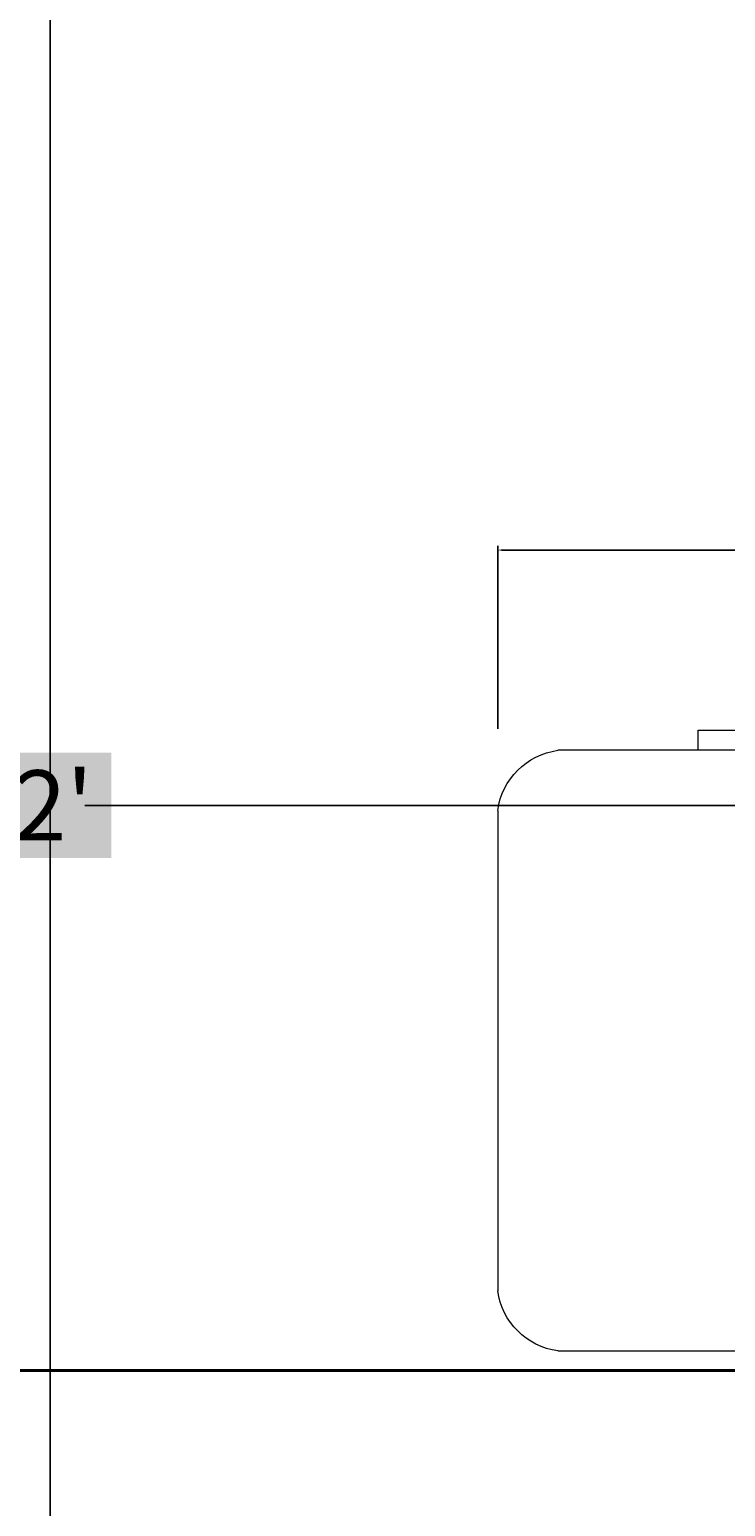
# Model space of a CAD drawing. Units: inches. Extents: x -301 to 715, y -607 to 364.
# Tile 77 of 141: x -123 to -94, y -73 to -10. Entities that reach past the tile are written whole.
import ezdxf

# ---------------------------------------------------------------- set-up
doc = ezdxf.new("R2010")
doc.units = ezdxf.units.IN
doc.header["$MEASUREMENT"] = 0
for name, color, linetype, lineweight in [('A-ANNO-DIMS', 2, 'Continuous', 18), ('A-FURN', 8, 'Continuous', 18), ('A-WALL', 3, 'Continuous', 40)]:
    doc.layers.add(name, color=color, linetype=linetype, lineweight=lineweight)
doc.styles.get("Standard").update_dxf_attribs({"font": 'arial.ttf'})
doc.dimstyles.get("Standard").update_dxf_attribs({"dimtxt": 0.18, "dimasz": 0.18, "dimexe": 0.18, "dimexo": 0.0625, "dimgap": 0.09, "dimtad": 0, "dimtih": 1, "dimtoh": 1, "dimdec": 1, "dimzin": 0, "dimdsep": 46, "dimlunit": 4, "dimtxsty": 'Standard', "dimcen": 0.09, "dimclrd": 3, "dimclre": 4, "dimclrt": 6, "dimadec": 0, "dimazin": 0, "dimtfac": 1, "dimtdec": 1, "dimtofl": 0, "dimtmove": 0, "dimatfit": 3, "dimfxl": 1, "dimtfill": 2, "dimtfillclr": 51, "dimtolj": 1, "dimtzin": 0, "dimarcsym": 0})

# ---------------------------------------------------------------- blocks, each defined once
blk = doc.blocks.new('Desk - 30 x 60 in.')
for p, q in [((-26.999995, 0), (26.999995, 0)), ((-29.999995, -27), (-29.999995, -3)), ((29.999995, -3), (29.999995, -27)), ((26.999995, -30), (-26.999995, -30)), ((-20.000005, -30), (-20.000005, -31)), ((-16.000005, -31), (-16.000005, -30)), ((15.999995, -31), (15.999995, -30)), ((19.999995, -30), (19.999995, -31)), ((-20.000005, -31), (-16.000005, -31)), ((19.999995, -31), (15.999995, -31))]:
    blk.add_line(p, q)
for centre, start, end in [((-26.499995, -3.5), 98.1301, 171.8699), ((26.499995, -3.5), 8.130102, 81.8699), ((-26.499995, -26.5), 188.1301, 261.8699), ((26.499995, -26.5), 278.1301, 351.8699)]:
    blk.add_arc(centre, 3.535534, start, end)
blk = doc.blocks.new('*D57')
at = {"layer": 'A-ANNO-DIMS', "color": 0, "lineweight": -2, "transparency": 16777216}
for p, q in [((-195.603, -67.255), (-195.603, -42.99)), ((-190.603, -43.17), (-126.098, -43.17)), ((-56.603, -43.17), (-121.109, -43.17)), ((-51.603, -67.255), (-51.603, -42.99))]:
    blk.add_line(p, q, dxfattribs=at)
at = {"layer": 'A-ANNO-DIMS', "color": 0, "transparency": 16777216}
for points in [[(-190.603, -42.336), (-190.603, -44.003), (-195.603, -43.17)], [(-56.603, -42.336), (-56.603, -44.003), (-51.603, -43.17)]]:
    blk.add_solid(points, dxfattribs=at)
at = {"layer": 'Defpoints', "color": 0, "transparency": 16777216}
for p in [(-51.603, -43.17), (-195.603, -67.318), (-51.603, -67.318)]:
    blk.add_point(p, dxfattribs=at)
at = {"layer": 'A-ANNO-DIMS', "color": 0, "transparency": 16777216, "insert": (-123.603, -43.17), "char_height": 3, "attachment_point": 5, "bg_fill": 1, "box_fill_scale": 1.25, "bg_fill_color": 51, "bg_fill_transparency": 0}
blk.add_mtext("\\A1;12'", dxfattribs=at)
blk = doc.blocks.new('*D114')
at = {"layer": 'A-ANNO-DIMS', "color": 4, "lineweight": -2, "transparency": 16777216}
for p, q in [((-103.477, -39.895), (-103.477, -32.076)), ((-52.128, -39.895), (-52.128, -32.076))]:
    blk.add_line(p, q, dxfattribs=at)
at = {"layer": 'A-ANNO-DIMS', "color": 3, "lineweight": -2, "transparency": 16777216}
for p, q in [((-103.297, -32.256), (-79.024, -32.256)), ((-52.308, -32.256), (-76.581, -32.256))]:
    blk.add_line(p, q, dxfattribs=at)
at = {"layer": 'A-ANNO-DIMS', "color": 3, "transparency": 16777216}
for points in [[(-103.297, -32.226), (-103.297, -32.286), (-103.477, -32.256)], [(-52.308, -32.226), (-52.308, -32.286), (-52.128, -32.256)]]:
    blk.add_solid(points, dxfattribs=at)
at = {"layer": 'Defpoints', "color": 0, "transparency": 16777216}
for p in [(-52.128, -32.256), (-103.477, -39.958), (-52.128, -39.958)]:
    blk.add_point(p, dxfattribs=at)
at = {"layer": 'A-ANNO-DIMS', "color": 6, "transparency": 16777216, "insert": (-77.803, -32.256), "char_height": 0.18, "attachment_point": 5, "bg_fill": 1, "box_fill_scale": 1.25, "bg_fill_color": 51, "bg_fill_transparency": 0}
blk.add_mtext('\\A1;DESK 4\'-3 1/2" TYP.', dxfattribs=at)
blk = doc.blocks.new('*D151')
at = {"layer": 'A-ANNO-DIMS', "color": 4, "lineweight": -2, "transparency": 16777216}
for p, q in [((-204.603, -223.755), (-204.603, 359.612)), ((-45.603, -214.755), (-45.603, 359.612))]:
    blk.add_line(p, q, dxfattribs=at)
at = {"layer": 'A-ANNO-DIMS', "color": 3, "lineweight": -2, "transparency": 16777216}
for p, q in [((-204.423, 359.432), (-125.494, 359.432)), ((-45.783, 359.432), (-124.713, 359.432))]:
    blk.add_line(p, q, dxfattribs=at)
at = {"layer": 'A-ANNO-DIMS', "color": 3, "transparency": 16777216}
for points in [[(-204.423, 359.462), (-204.423, 359.402), (-204.603, 359.432)], [(-45.783, 359.462), (-45.783, 359.402), (-45.603, 359.432)]]:
    blk.add_solid(points, dxfattribs=at)
at = {"layer": 'Defpoints', "color": 0, "transparency": 16777216}
for p in [(-45.603, 359.432), (-45.603, -214.818), (-204.603, -223.818)]:
    blk.add_point(p, dxfattribs=at)
at = {"layer": 'A-ANNO-DIMS', "color": 6, "transparency": 16777216, "insert": (-125.103, 359.432), "char_height": 0.18, "attachment_point": 5, "bg_fill": 1, "box_fill_scale": 1.25, "bg_fill_color": 51, "bg_fill_transparency": 0}
blk.add_mtext('\\A1;13\'-3"', dxfattribs=at)
blk = doc.blocks.new('*D158')
at = {"layer": 'A-ANNO-DIMS', "color": 4, "lineweight": -2, "transparency": 16777216}
for p, q in [((-122.603, 221.62), (-122.603, -296.865)), ((-50.603, 221.62), (-50.603, -296.865))]:
    blk.add_line(p, q, dxfattribs=at)
at = {"layer": 'A-ANNO-DIMS', "color": 3, "lineweight": -2, "transparency": 16777216}
for p, q in [((-122.423, -296.685), (-86.933, -296.685)), ((-50.783, -296.685), (-86.274, -296.685))]:
    blk.add_line(p, q, dxfattribs=at)
at = {"layer": 'A-ANNO-DIMS', "color": 3, "transparency": 16777216}
for points in [[(-122.423, -296.655), (-122.423, -296.715), (-122.603, -296.685)], [(-50.783, -296.655), (-50.783, -296.715), (-50.603, -296.685)]]:
    blk.add_solid(points, dxfattribs=at)
at = {"layer": 'Defpoints', "color": 0, "transparency": 16777216}
for p in [(-122.603, 221.682), (-50.603, 221.682), (-50.603, -296.685)]:
    blk.add_point(p, dxfattribs=at)
at = {"layer": 'A-ANNO-DIMS', "color": 6, "transparency": 16777216, "insert": (-86.603, -296.685), "char_height": 0.18, "attachment_point": 5, "bg_fill": 1, "box_fill_scale": 1.25, "bg_fill_color": 51, "bg_fill_transparency": 0}
blk.add_mtext('\\A1;6\'-0"', dxfattribs=at)

msp = doc.modelspace()

# ---------------------------------------------------------------- linework, layer by layer
at = {"layer": 'A-WALL'}
msp.add_line((-195.603, -67.318), (-51.603, -67.318), dxfattribs=at)

# ---------------------------------------------------------------- block references
at = {"layer": 'A-FURN', "xscale": -0.8558048107780498, "yscale": 0.8558048107780498, "zscale": 0.8558048107780498, "rotation": 180}
msp.add_blockref('Desk - 30 x 60 in.', (-77.803, -66.488), dxfattribs=at)

# ---------------------------------------------------------------- dimensions: what is measured, and where the dimension line sits
at = {"layer": 'A-ANNO-DIMS'}
for base, p1, p2, override, picture, middle in [((-45.603, 359.432), (-204.603, -223.818), (-45.603, -214.818), {"dimdec": 1, "dimlfac": 1, "dimrnd": 0, "dimzin": 1, "dimdsep": 46, "dimlunit": 4, "dimfrac": 2}, '*D151', (-125.103, 359.432)), ((-50.603, -296.685), (-122.603, 221.682), (-50.603, 221.682), {"dimdec": 1, "dimlfac": 1, "dimrnd": 0, "dimzin": 1, "dimdsep": 46, "dimlunit": 4, "dimfrac": 2}, '*D158', (-86.603, -296.685)), ((-51.603, -43.17), (-195.603, -67.318), (-51.603, -67.318), {"dimtxt": 3, "dimasz": 5, "dimclrd": 0, "dimclre": 0, "dimclrt": 0}, '*D57', (-123.603, -43.17))]:
    dim = msp.add_linear_dim(base=base, p1=p1, p2=p2, dimstyle='Standard', override=override, dxfattribs=at)
    dim.commit()
    dim.dimension.update_dxf_attribs({"geometry": picture, "text_midpoint": middle})
dim = msp.add_linear_dim(base=(-52.128, -32.256), p1=(-103.477, -39.958), p2=(-52.128, -39.958), text='DESK <> TYP.', dimstyle='Standard', override={"dimdec": 1, "dimlfac": 1, "dimrnd": 0, "dimzin": 1, "dimdsep": 46, "dimlunit": 4, "dimfrac": 2}, dxfattribs=at)
dim.commit()
dim.dimension.update_dxf_attribs({"geometry": '*D114', "text_midpoint": (-77.803, -32.256)})

doc.saveas('drawing.dxf')
